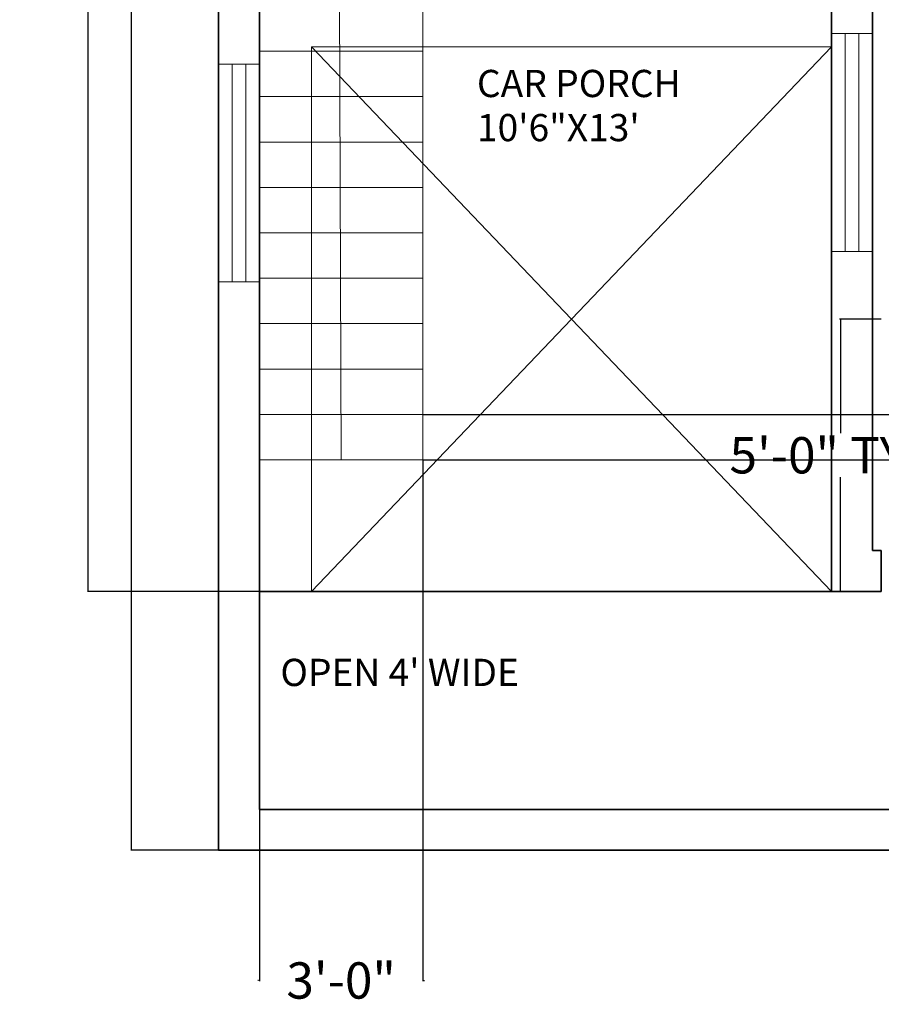
# Model space of a CAD drawing. Units: inches. Extents: x 125 to 976, y 231 to 853.
# Tile 1 of 16: x 134 to 324, y 238 to 455. Entities that reach past the tile are written whole.
import ezdxf

# ---------------------------------------------------------------- set-up
doc = ezdxf.new("R2010")
doc.units = ezdxf.units.IN
doc.header["$MEASUREMENT"] = 0
for name, color, linetype, lineweight in [('A-ANNO-DIMS', 2, 'Continuous', 18), ('A-AREA-IDEN', 7, 'Continuous', 18), ('A-FLOR', 8, 'Continuous', 18), ('A-FLOR-STRS', 7, 'Continuous', 18), ('A-GLAZ', 4, 'Continuous', 18), ('A-WALL', 7, 'Continuous', 35)]:
    doc.layers.add(name, color=color, linetype=linetype, lineweight=lineweight)
doc.styles.get("Standard").update_dxf_attribs({"font": 'italic8.shx'})
doc.dimstyles.get("Standard").update_dxf_attribs({"dimtxt": 8, "dimasz": 0.18, "dimexe": 0.18, "dimexo": 0.0625, "dimgap": 0.09, "dimtad": 0, "dimtih": 1, "dimtoh": 1, "dimdec": 4, "dimzin": 0, "dimdsep": 46, "dimlunit": 3, "dimtxsty": 'Standard', "dimcen": 0.09, "dimclrt": 4, "dimadec": 0, "dimazin": 0, "dimtfac": 1, "dimtdec": 4, "dimtofl": 0, "dimtmove": 0, "dimatfit": 3, "dimfxl": 1, "dimtolj": 1, "dimtzin": 0, "dimarcsym": 0})

# ---------------------------------------------------------------- blocks, each defined once
blk = doc.blocks.new('*D4')
at = {"layer": 'A-ANNO-DIMS', "color": 0, "lineweight": -2, "transparency": 16777216}
for p, q in [((177.52, 812.1), (158.26, 812.1)), ((158.44, 811.92), (158.44, 546.96)), ((158.44, 272.28), (158.44, 537.25)), ((177.52, 272.1), (158.26, 272.1))]:
    blk.add_line(p, q, dxfattribs=at)
at = {"layer": 'A-ANNO-DIMS', "color": 0, "transparency": 16777216}
for points in [[(158.41, 811.92), (158.47, 811.92), (158.44, 812.1)], [(158.41, 272.28), (158.47, 272.28), (158.44, 272.1)]]:
    blk.add_solid(points, dxfattribs=at)
at = {"layer": 'Defpoints', "color": 0, "transparency": 16777216}
for p in [(177.58, 812.1), (158.44, 272.1), (177.58, 272.1)]:
    blk.add_point(p, dxfattribs=at)
at = {"layer": 'A-ANNO-DIMS', "color": 0, "transparency": 16777216, "insert": (158.44, 542.1), "char_height": 8, "attachment_point": 5}
blk.add_mtext("\\A1;45'", dxfattribs=at)
blk = doc.blocks.new('WINDOW-48IN')
for p, q in [((0, 0), (0, 48)), ((0, 48), (9, 48)), ((3, 0), (3, 48)), ((6, 0), (6, 48)), ((9, 48), (9, 0)), ((9, 0), (0, 0))]:
    blk.add_line(p, q)
blk = doc.blocks.new('*D55')
at = {"layer": 'A-ANNO-DIMS', "color": 0, "lineweight": -2, "transparency": 16777216}
for p, q in [((323.45, 389.1), (314.33, 389.1)), ((314.51, 388.92), (314.51, 363.96)), ((314.51, 329.28), (314.51, 354.25)), ((323.45, 329.1), (314.33, 329.1))]:
    blk.add_line(p, q, dxfattribs=at)
at = {"layer": 'A-ANNO-DIMS', "color": 0, "transparency": 16777216}
for points in [[(314.48, 388.92), (314.54, 388.92), (314.51, 389.1)], [(314.48, 329.28), (314.54, 329.28), (314.51, 329.1)]]:
    blk.add_solid(points, dxfattribs=at)
at = {"layer": 'Defpoints', "color": 0, "transparency": 16777216}
for p in [(314.51, 389.1), (323.51, 389.1), (323.51, 329.1)]:
    blk.add_point(p, dxfattribs=at)
at = {"layer": 'A-ANNO-DIMS', "color": 4, "transparency": 16777216, "insert": (314.51, 359.1), "char_height": 8, "attachment_point": 5}
blk.add_mtext('\\A1;5\'-0" TYP.', dxfattribs=at)
blk = doc.blocks.new('*D56')
at = {"layer": 'A-ANNO-DIMS', "color": 0, "lineweight": -2, "transparency": 16777216}
for p, q in [((177.52, 812.1), (148.7, 812.1)), ((148.88, 811.92), (148.88, 575.46)), ((148.88, 329.28), (148.88, 565.75)), ((186.52, 329.1), (148.7, 329.1))]:
    blk.add_line(p, q, dxfattribs=at)
at = {"layer": 'A-ANNO-DIMS', "color": 0, "transparency": 16777216}
for points in [[(148.85, 811.92), (148.91, 811.92), (148.88, 812.1)], [(148.85, 329.28), (148.91, 329.28), (148.88, 329.1)]]:
    blk.add_solid(points, dxfattribs=at)
at = {"layer": 'Defpoints', "color": 0, "transparency": 16777216}
for p in [(148.88, 812.1), (177.58, 812.1), (186.58, 329.1)]:
    blk.add_point(p, dxfattribs=at)
at = {"layer": 'A-ANNO-DIMS', "color": 4, "transparency": 16777216, "insert": (148.88, 570.6), "char_height": 8, "attachment_point": 5}
blk.add_mtext('\\A1;40\'-3"', dxfattribs=at)
blk = doc.blocks.new('*D58')
at = {"layer": 'A-ANNO-DIMS', "color": 0, "lineweight": -2, "transparency": 16777216}
for p, q in [((186.579198, 358.042246), (186.579198, 243.224746)), ((222.579198, 358.042246), (222.579198, 243.224746)), ((186.399198, 243.404746), (186.219198, 243.404746)), ((222.759198, 243.404746), (222.939198, 243.404746))]:
    blk.add_line(p, q, dxfattribs=at)
at = {"layer": 'A-ANNO-DIMS', "color": 0, "transparency": 16777216}
for points in [[(186.399198, 243.434746), (186.399198, 243.374746), (186.579198, 243.404746)], [(222.759198, 243.434746), (222.759198, 243.374746), (222.579198, 243.404746)]]:
    blk.add_solid(points, dxfattribs=at)
at = {"layer": 'Defpoints', "color": 0, "transparency": 16777216}
for p in [(186.579198, 358.104746), (222.579198, 358.104746), (222.579198, 243.404746)]:
    blk.add_point(p, dxfattribs=at)
at = {"layer": 'A-ANNO-DIMS', "color": 4, "transparency": 16777216, "insert": (204.579198, 243.404746), "char_height": 8, "attachment_point": 5}
blk.add_mtext('\\A1;3\'-0"', dxfattribs=at)
blk = doc.blocks.new('*D59')
at = {"layer": 'A-ANNO-DIMS', "color": 0, "lineweight": -2, "transparency": 16777216}
for p, q in [((222.641698, 368.104746), (494.459198, 368.104746)), ((494.279198, 368.284746), (494.279198, 368.464746)), ((222.641698, 358.104746), (494.459198, 358.104746)), ((494.279198, 357.924746), (494.279198, 357.744746))]:
    blk.add_line(p, q, dxfattribs=at)
at = {"layer": 'A-ANNO-DIMS', "color": 0, "transparency": 16777216}
for points in [[(494.249198, 368.284746), (494.309198, 368.284746), (494.279198, 368.104746)], [(494.249198, 357.924746), (494.309198, 357.924746), (494.279198, 358.104746)]]:
    blk.add_solid(points, dxfattribs=at)
at = {"layer": 'Defpoints', "color": 0, "transparency": 16777216}
for p in [(222.579198, 368.104746), (494.279198, 368.104746), (222.579198, 358.104746)]:
    blk.add_point(p, dxfattribs=at)
at = {"layer": 'A-ANNO-DIMS', "color": 4, "transparency": 16777216, "insert": (494.279198, 363.104746), "char_height": 8, "attachment_point": 5}
blk.add_mtext('\\A1;0\'-10"', dxfattribs=at)

msp = doc.modelspace()

# ---------------------------------------------------------------- linework, layer by layer
at = {"layer": 'A-FLOR'}
for p, q in [((198.05682, 329.10475), (198.05682, 449.10475)), ((198.05682, 449.10475), (312.5792, 449.10475)), ((312.5792, 449.10475), (198.05682, 329.10475)), ((312.5792, 329.10475), (198.05682, 449.10475))]:
    msp.add_line(p, q, dxfattribs=at)
at = {"layer": 'A-FLOR-STRS'}
for p, q in [((222.5792, 494.10475), (222.5792, 358.10475)), ((204.18906, 476.10475), (204.5792, 358.10475)), ((222.5792, 448.10475), (186.5792, 448.10475)), ((222.5792, 438.10475), (186.5792, 438.10475)), ((222.5792, 428.10475), (186.5792, 428.10475)), ((222.5792, 418.10475), (186.5792, 418.10475)), ((222.5792, 408.10475), (186.5792, 408.10475)), ((222.5792, 398.10475), (186.5792, 398.10475)), ((222.5792, 388.10475), (186.5792, 388.10475)), ((222.5792, 378.10475), (186.5792, 378.10475)), ((222.5792, 368.10475), (186.5792, 368.10475)), ((222.5792, 358.10475), (186.5792, 358.10475))]:
    msp.add_line(p, q, dxfattribs=at)
at = {"layer": 'A-WALL'}
for p, q in [((186.5792, 494.10475), (186.5792, 281.10475)), ((312.5792, 494.10475), (312.5792, 329.10475)), ((312.5792, 338.10475), (312.5792, 494.10475)), ((321.5792, 494.10475), (321.5792, 338.10475)), ((321.5792, 338.10475), (323.51392, 338.10475)), ((323.51392, 338.10475), (323.51392, 329.10475)), ((186.5792, 329.10475), (323.51392, 329.10475)), ((186.5792, 281.10475), (456.5792, 281.10475))]:
    msp.add_line(p, q, dxfattribs=at)
msp.add_lwpolyline([(177.5792, 272.10475), (465.5792, 272.10475), (465.5792, 812.10475), (177.5792, 812.10475)], close=True, dxfattribs=at)

# ---------------------------------------------------------------- block references
at = {"layer": 'A-GLAZ'}
for p in [(312.57633, 403.9997), (177.57633, 397.29145)]:
    msp.add_blockref('WINDOW-48IN', p, dxfattribs=at)

# ---------------------------------------------------------------- texts
at = {"layer": 'A-AREA-IDEN'}
for s, p in [('CAR PORCH', (234.47585, 438.00188)), ('10\'6"X13\'', (234.47585, 428.2876)), ("OPEN 4' WIDE", (191.19577, 308.26875))]:
    msp.add_text(s, height=6, dxfattribs=at).set_placement(p)

# ---------------------------------------------------------------- dimensions: what is measured, and where the dimension line sits
at = {"layer": 'A-ANNO-DIMS'}
for base, p1, p2, override, picture, middle in [((148.8792, 812.10475), (186.5792, 329.10475), (177.5792, 812.10475), {"dimdec": 1, "dimlfac": 1, "dimrnd": 0, "dimzin": 1, "dimdsep": 46, "dimlunit": 4, "dimfrac": 2}, '*D56', (148.8792, 570.60475)), ((158.44384, 272.10475), (177.5792, 812.10475), (177.5792, 272.10475), {"dimclrd": 0, "dimclre": 0, "dimclrt": 0}, '*D4', (158.44384, 542.10475)), ((494.2792, 368.10475), (222.5792, 358.10475), (222.5792, 368.10475), {"dimdec": 1, "dimlfac": 1, "dimrnd": 0, "dimzin": 1, "dimdsep": 46, "dimlunit": 4, "dimfrac": 2}, '*D59', (494.2792, 363.10475))]:
    dim = msp.add_linear_dim(base=base, p1=p1, p2=p2, angle=90, dimstyle='Standard', override=override, dxfattribs=at)
    dim.commit()
    dim.dimension.update_dxf_attribs({"geometry": picture, "text_midpoint": middle})
dim = msp.add_linear_dim(base=(314.51392, 389.10475), p1=(323.51392, 329.10475), p2=(323.51392, 389.10475), angle=90, text='<> TYP.', dimstyle='Standard', override={"dimdec": 1, "dimlfac": 1, "dimrnd": 0, "dimzin": 1, "dimdsep": 46, "dimlunit": 4, "dimfrac": 2}, dxfattribs=at)
dim.commit()
dim.dimension.update_dxf_attribs({"geometry": '*D55', "text_midpoint": (314.51392, 359.10475)})
dim = msp.add_linear_dim(base=(222.5792, 243.40475), p1=(186.5792, 358.10475), p2=(222.5792, 358.10475), dimstyle='Standard', override={"dimdec": 1, "dimlfac": 1, "dimrnd": 0, "dimzin": 1, "dimdsep": 46, "dimlunit": 4, "dimfrac": 2}, dxfattribs=at)
dim.commit()
dim.dimension.update_dxf_attribs({"geometry": '*D58', "text_midpoint": (204.5792, 243.40475)})

doc.saveas('drawing.dxf')
